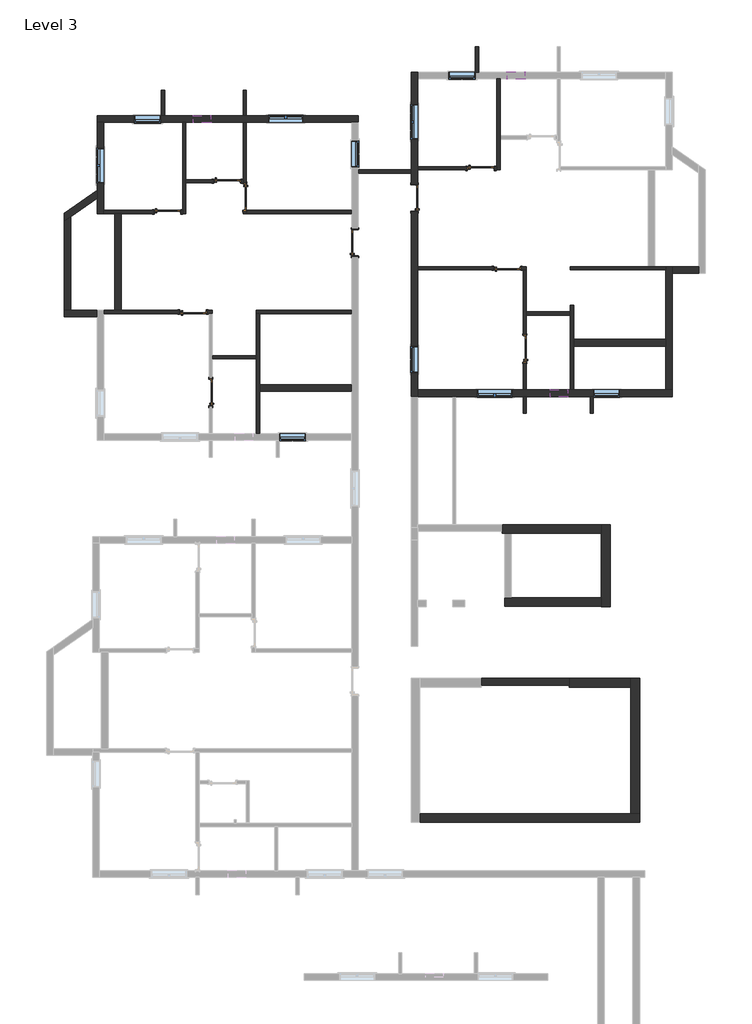
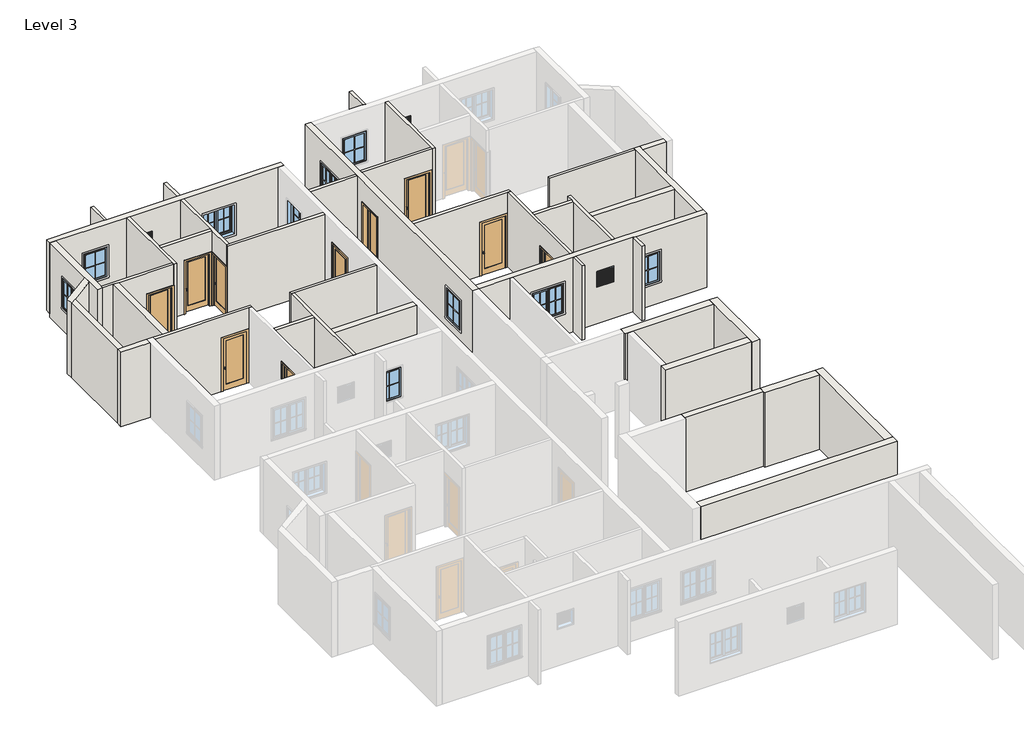
# One storey, part 5 of 7: 41 walls, 13 windows, 10 doors.
# Revit data of these elements (continued)
# Element 55 (IfcWindow, "Window-Awning-Single : 36\" x 48\"") (continued)
#   Interior Wall Closure = 0' - 2 1/4"
#   Frame Extension = 0' - 0 1/4"
#   Exterior Wall Closure = 0' - 1 1/4"
#   Interior Trim Visibility = yes
#   Exterior Trim Visibility = yes
#   Phase Created = New Construction
#   Materials on its faces: "Wood - Stained", "Glass", "Clad - White"
# Element 56 (IfcWindow, "Window-Awning-Single : 36\" x 48\"")
#   Mark = "24"
#   Window Inset = 0' - 0"
#   Interior Wall Closure = 0' - 2 1/4"
#   Frame Extension = 0' - 0 1/4"
#   Exterior Wall Closure = 0' - 1 1/4"
#   Interior Trim Visibility = yes
#   Exterior Trim Visibility = yes
#   Phase Created = New Construction
#   Materials on its faces: "Wood - Stained", "Glass", "Clad - White"
# Element 57 (IfcWindow, "Window-Awning-Single : 36\" x 48\"")
#   Mark = "25"
#   Window Inset = 0' - 0"
#   Interior Wall Closure = 0' - 2 1/4"
#   Frame Extension = 0' - 0 1/4"
#   Exterior Wall Closure = 0' - 1 1/4"
#   Interior Trim Visibility = yes
#   Exterior Trim Visibility = yes
#   Phase Created = New Construction
#   Materials on its faces: "Wood - Stained", "Glass", "Clad - White"
# Element 58 (IfcWindow, "Window-Casement-Double : 4' x 4'")
#   Mark = "34"
#   Window Inset = 0' - 0"
#   Interior Wall Closure = 0' - 2 1/4"
#   Frame Extension = 0' - 0 1/4"
#   Exterior Wall Closure = 0' - 1 1/4"
#   Interior Trim Visibility = yes
#   Exterior Trim Visibility = yes
#   Phase Created = New Construction
#   Materials on its faces: "Wood - Stained", "Glass", "Clad - White"
# Element 59 (IfcWindow, "Window-Casement-Double : 4' x 4'")
#   Mark = "35"
#   Window Inset = 0' - 0"
#   Interior Wall Closure = 0' - 2 1/4"
#   Frame Extension = 0' - 0 1/4"
#   Exterior Wall Closure = 0' - 1 1/4"
#   Interior Trim Visibility = yes
#   Exterior Trim Visibility = yes
#   Phase Created = New Construction
#   Materials on its faces: "Wood - Stained", "Glass", "Clad - White"
# Element 60 (IfcWindow, "Window-Casement-Double : 4' x 4'")
#   Mark = "37"
#   Window Inset = 0' - 0"
#   Interior Wall Closure = 0' - 2 1/4"
#   Frame Extension = 0' - 0 1/4"
#   Exterior Wall Closure = 0' - 1 1/4"
#   Interior Trim Visibility = yes
#   Exterior Trim Visibility = yes
#   Phase Created = New Construction
#   Materials on its faces: "Wood - Stained", "Glass", "Clad - White"
# Element 61 (IfcWindow, "Window-Casement-Double : 4' x 4'")
#   Mark = "39"
#   Window Inset = 0' - 0"
#   Interior Wall Closure = 0' - 2 1/4"
#   Frame Extension = 0' - 0 1/4"
#   Exterior Wall Closure = 0' - 1 1/4"
#   Interior Trim Visibility = yes
#   Exterior Trim Visibility = yes
#   Phase Created = New Construction
#   Materials on its faces: "Wood - Stained", "Glass", "Clad - White"
# Element 62 (IfcWindow, "Window-Louvers : 24\" x 24\"")
#   Mark = "1"
#   Blade Width = 1' - 10 1/2"
#   Phase Created = New Construction
#   Materials on its faces: "Birch"
# Element 63 (IfcWindow, "Window-Louvers : 24\" x 24\"")
#   Mark = "3"
#   Blade Width = 1' - 10 1/2"
#   Phase Created = New Construction
#   Materials on its faces: "Birch"
# Element 64 (IfcWindow, "Window-Louvers : 24\" x 24\"")
#   Mark = "4"
#   Blade Width = 1' - 10 1/2"
#   Phase Created = New Construction
#   Materials on its faces: "Birch"
# Materials
#   "Cherry": class "Wood", colour RGB 226 177 128, transparency 0, Description = "Prunus Serotina", Cost = 0
#   "Aluminum": class "Metal", colour RGB 247 247 247, transparency 0, Description = "Aluminum 6061", Cost = 0
#   "Wood - Stained": class "Wood", colour RGB 224 178 126, transparency 0, Cost = 0
#   "Glass": class "Glass", colour RGB 0 128 192, transparency 0.75, Description = "Soda Lime Glass", Cost = 0
#   "Clad - White": class "Wood", colour RGB 242 242 238, transparency 0, Cost = 0
#   "Birch": class "Wood", colour RGB 224 178 126, transparency 0, Description = "Betula Alleghaniensis", Cost = 0
#   "Default Wall": colour RGB 128 128 128, transparency 0, Cost = 0
